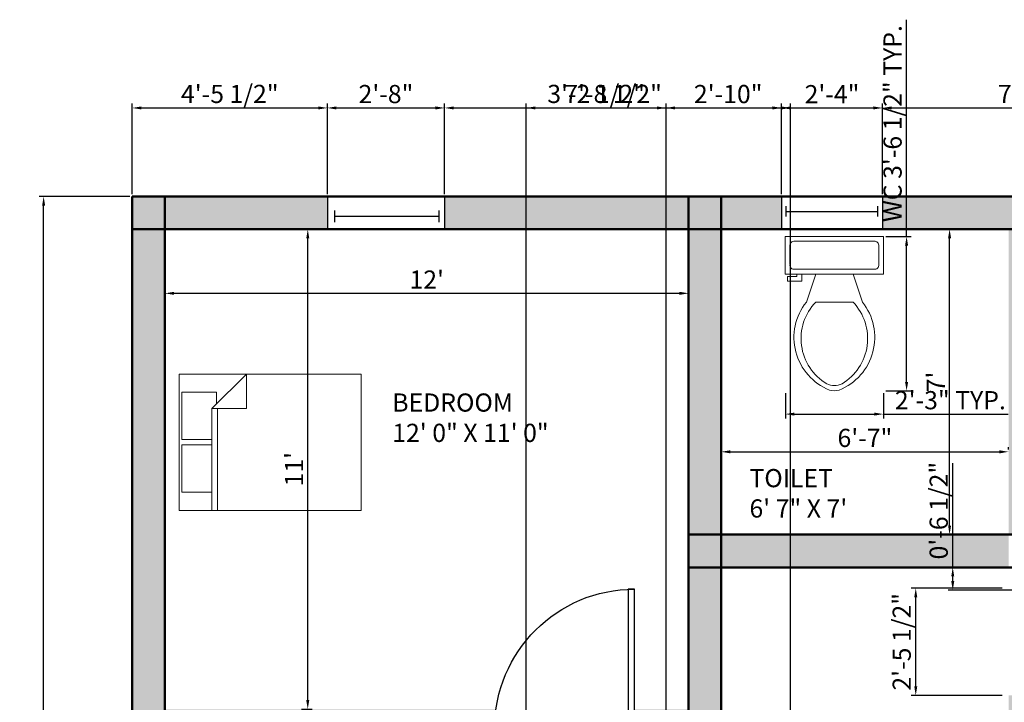
# Model space of a CAD drawing. Units: millimetres. Extents: x 3012 to 3478, y 929 to 1463.
# Tile 3 of 4: x 3012 to 3283, y 1275 to 1463. Entities that reach past the tile are written whole.
import ezdxf

# ---------------------------------------------------------------- set-up
doc = ezdxf.new("R2010")
doc.units = ezdxf.units.MM
for name, color, linetype, lineweight in [('A-ANNO-DIMS', 50, 'Continuous', 18), ('A-AREA-IDEN', 170, 'Continuous', 25), ('A-FLOR-FIXT', 9, 'Continuous', 18), ('A-WALL-PATT', 252, 'Continuous', 13), ('doors', 130, 'Continuous', 25), ('furniture', 80, 'Continuous', 18), ('walls', 10, 'Continuous', 50), ('windows', 40, 'Continuous', 25)]:
    doc.layers.add(name, color=color, linetype=linetype, lineweight=lineweight)
doc.styles.get("Standard").update_dxf_attribs({"font": 'arial.ttf'})
doc.dimstyles.new('ISO-25', dxfattribs={"dimtxt": 5, "dimasz": 2.5, "dimexe": 1.25, "dimexo": 0.625, "dimtad": 1, "dimdec": 0, "dimlunit": 3, "dimtxsty": 'Standard', "dimcen": 2.5, "dimadec": 0, "dimazin": 0, "dimtfac": 1, "dimtdec": 0, "dimtmove": 0, "dimatfit": 3, "dimfxl": 1, "dimarcsym": 0})

# ---------------------------------------------------------------- blocks, each defined once
blk = doc.blocks.new('*U2')
for p, q in [((0, 0), (0, -6)), ((40, 0), (40, -6))]:
    blk.add_line(p, q)
blk.add_lwpolyline([(0, 0), (0, 40), (1.75, 40), (1.75, 0)], close=True)
blk.add_arc((0, 0), 40, 0, 90)
blk = doc.blocks.new('*U4')
for p, q in [((0, 4), (0, 0)), ((36, 4), (36, 0)), ((0, 2), (36, 2))]:
    blk.add_line(p, q)
blk = doc.blocks.new('*U5')
for p, q in [((0, 4), (0, 0)), ((36, 4), (36, 0)), ((0, 2), (36, 2))]:
    blk.add_line(p, q)
blk = doc.blocks.new('Bed - Queen')
for p, q in [((0, -80.00003), (0, 0)), ((0, 0), (59.99999, 0)), ((59.99999, 0), (59.99999, -80.00003)), ((7.99999, -1.2), (28.79998, -1.2)), ((7.99999, -14.4), (7.99999, -1.2)), ((28.79998, -1.2), (28.79998, -14.4)), ((31.19999, -1.2), (51.99999, -1.2)), ((31.19999, -14.4), (31.19999, -1.2)), ((51.99999, -1.2), (51.99999, -16.4)), ((0, -14.4), (44.8, -14.4)), ((44.8, -16.8), (0, -16.8)), ((59.99999, -29.6), (44.8, -14.4)), ((44.8, -14.4), (44.8, -29.6)), ((51.99999, -16.4), (46.79936, -16.4)), ((44.8, -29.6), (59.99999, -29.6)), ((59.99999, -80.00003), (0, -80.00003))]:
    blk.add_line(p, q)
blk = doc.blocks.new('Toilet - top')
for p, q in [((9.5, -6), (9.5, -2)), ((-8, -8.5), (-8, -8)), ((-7, -8), (-7, -9.5)), ((-4, -8), (-6, -14)), ((4, -8), (6, -14)), ((-10, -8.5), (-8, -8.5)), ((-10, -9.5), (-10, -8.5)), ((-7, -9.5), (-10, -9.5)), ((4, -14), (-4, -14))]:
    blk.add_line(p, q)
blk.add_lwpolyline([(10.5, -8), (10.5, 0), (-10.5, 0), (-10.5, -8)], close=True)
for points in [[(-9.5, -2), (-9.5, -6)], [(8.5, -1), (-8.5, -1)], [(-8.5, -7), (8.5, -7)]]:
    blk.add_lwpolyline(points)
for centre, radius, start, end in [((-8.62, -1.88), 0.884, 81.8699, 188.1301), ((8.62, -1.88), 0.884, 351.8699, 98.1301), ((-8.62, -6.12), 0.884, 171.8699, 278.1301), ((8.62, -6.12), 0.884, 261.8699, 8.1301), ((3.52, -21.58), 12.17, 141.4691, 247.9714), ((4.2, -21.82), 11.33, 136.3677, 238.9468), ((-3.52, -21.58), 12.17, 292.0284, 38.5307), ((-4.2, -21.82), 11.33, 301.053, 43.6321), ((0, -27.88), 4, 245.7318, 294.2682), ((0, -29), 4, 254.8605, 285.1395)]:
    blk.add_arc(centre, radius, start, end)
blk = doc.blocks.new('*D12')
at = {"layer": 'A-ANNO-DIMS', "color": 0, "lineweight": -2, "transparency": 16777216}
for p, q in [((3052.21, 1392.44), (3052.21, 1386.56)), ((3196.21, 1392.44), (3196.21, 1386.56)), ((3054.71, 1387.81), (3193.71, 1387.81))]:
    blk.add_line(p, q, dxfattribs=at)
at = {"layer": 'A-ANNO-DIMS', "color": 0, "transparency": 16777216}
for points in [[(3054.71, 1388.22), (3054.71, 1387.39), (3052.21, 1387.81)], [(3193.71, 1388.22), (3193.71, 1387.39), (3196.21, 1387.81)]]:
    blk.add_solid(points, dxfattribs=at)
at = {"layer": 'Defpoints', "color": 0, "transparency": 16777216}
for p in [(3052.21, 1393.06), (3196.21, 1393.06), (3196.21, 1387.81)]:
    blk.add_point(p, dxfattribs=at)
at = {"layer": 'A-ANNO-DIMS', "color": 0, "transparency": 16777216, "insert": (3124.21, 1390.94), "char_height": 5, "attachment_point": 5}
blk.add_mtext("12'", dxfattribs=at)
blk = doc.blocks.new('*D13')
at = {"layer": 'A-ANNO-DIMS', "color": 0, "lineweight": -2, "transparency": 16777216}
for p, q in [((3089.79, 1405.44), (3092.75, 1405.44)), ((3091.5, 1275.94), (3091.5, 1402.94)), ((3089.79, 1273.44), (3092.75, 1273.44))]:
    blk.add_line(p, q, dxfattribs=at)
at = {"layer": 'A-ANNO-DIMS', "color": 0, "transparency": 16777216}
for points in [[(3091.08, 1402.94), (3091.91, 1402.94), (3091.5, 1405.44)], [(3091.08, 1275.94), (3091.91, 1275.94), (3091.5, 1273.44)]]:
    blk.add_solid(points, dxfattribs=at)
at = {"layer": 'Defpoints', "color": 0, "transparency": 16777216}
for p in [(3089.17, 1405.44), (3091.5, 1405.44), (3089.17, 1273.44)]:
    blk.add_point(p, dxfattribs=at)
at = {"layer": 'A-ANNO-DIMS', "color": 0, "transparency": 16777216, "insert": (3088.36, 1339.44), "char_height": 5, "attachment_point": 5, "rotation": 90}
blk.add_mtext("11'", dxfattribs=at)
blk = doc.blocks.new('*D14')
at = {"layer": 'A-ANNO-DIMS', "color": 0, "lineweight": -2, "transparency": 16777216}
for p, q in [((3205.21, 1344.85), (3205.21, 1345.47)), ((3207.71, 1344.22), (3281.71, 1344.22)), ((3284.21, 1344.85), (3284.21, 1345.47))]:
    blk.add_line(p, q, dxfattribs=at)
at = {"layer": 'A-ANNO-DIMS', "color": 0, "transparency": 16777216}
for points in [[(3207.71, 1344.64), (3207.71, 1343.8), (3205.21, 1344.22)], [(3281.71, 1344.64), (3281.71, 1343.8), (3284.21, 1344.22)]]:
    blk.add_solid(points, dxfattribs=at)
at = {"layer": 'Defpoints', "color": 0, "transparency": 16777216}
for p in [(3205.21, 1344.22), (3284.21, 1344.22), (3284.21, 1344.22)]:
    blk.add_point(p, dxfattribs=at)
at = {"layer": 'A-ANNO-DIMS', "color": 0, "transparency": 16777216, "insert": (3244.71, 1347.4), "char_height": 5, "attachment_point": 5}
blk.add_mtext('6\'-7"', dxfattribs=at)
blk = doc.blocks.new('*D15')
at = {"layer": 'A-ANNO-DIMS', "color": 0, "lineweight": -2, "transparency": 16777216}
for p, q in [((3268.62, 1405.44), (3269.24, 1405.44)), ((3267.99, 1323.94), (3267.99, 1402.94)), ((3268.62, 1321.44), (3269.24, 1321.44))]:
    blk.add_line(p, q, dxfattribs=at)
at = {"layer": 'A-ANNO-DIMS', "color": 0, "transparency": 16777216}
for points in [[(3267.58, 1402.94), (3268.41, 1402.94), (3267.99, 1405.44)], [(3267.58, 1323.94), (3268.41, 1323.94), (3267.99, 1321.44)]]:
    blk.add_solid(points, dxfattribs=at)
at = {"layer": 'Defpoints', "color": 0, "transparency": 16777216}
for p in [(3267.99, 1405.44), (3267.99, 1405.44), (3267.99, 1321.44)]:
    blk.add_point(p, dxfattribs=at)
at = {"layer": 'A-ANNO-DIMS', "color": 0, "transparency": 16777216, "insert": (3264.87, 1363.44), "char_height": 5, "attachment_point": 5, "rotation": 90}
blk.add_mtext("7'", dxfattribs=at)
blk = doc.blocks.new('*D32')
at = {"layer": 'A-ANNO-DIMS', "color": 0, "lineweight": -2, "transparency": 16777216}
for p, q in [((3256.17, 1403.4), (3256.17, 1463.07)), ((3250.43, 1403.4), (3257.42, 1403.4)), ((3256.17, 1363.46), (3256.17, 1400.9)), ((3250.43, 1360.96), (3257.42, 1360.96))]:
    blk.add_line(p, q, dxfattribs=at)
at = {"layer": 'A-ANNO-DIMS', "color": 0, "transparency": 16777216}
for points in [[(3255.75, 1400.9), (3256.59, 1400.9), (3256.17, 1403.4)], [(3255.75, 1363.46), (3256.59, 1363.46), (3256.17, 1360.96)]]:
    blk.add_solid(points, dxfattribs=at)
at = {"layer": 'Defpoints', "color": 0, "transparency": 16777216}
for p in [(3249.8, 1403.4), (3256.17, 1403.4), (3249.8, 1360.96)]:
    blk.add_point(p, dxfattribs=at)
at = {"layer": 'A-ANNO-DIMS', "color": 0, "transparency": 16777216, "insert": (3252.96, 1434.49), "char_height": 5, "attachment_point": 5, "rotation": 90}
blk.add_mtext('WC 3\'-6 1/2" TYP.', dxfattribs=at)
blk = doc.blocks.new('*D33')
at = {"layer": 'A-ANNO-DIMS', "color": 0, "lineweight": -2, "transparency": 16777216}
for p, q in [((3222.83, 1360.33), (3222.83, 1353.34)), ((3249.8, 1360.33), (3249.8, 1353.34)), ((3225.33, 1354.59), (3247.3, 1354.59)), ((3249.8, 1354.59), (3284.11, 1354.59))]:
    blk.add_line(p, q, dxfattribs=at)
at = {"layer": 'A-ANNO-DIMS', "color": 0, "transparency": 16777216}
for points in [[(3225.33, 1355.01), (3225.33, 1354.17), (3222.83, 1354.59)], [(3247.3, 1355.01), (3247.3, 1354.17), (3249.8, 1354.59)]]:
    blk.add_solid(points, dxfattribs=at)
at = {"layer": 'Defpoints', "color": 0, "transparency": 16777216}
for p in [(3222.83, 1360.96), (3249.8, 1360.96), (3249.8, 1354.59)]:
    blk.add_point(p, dxfattribs=at)
at = {"layer": 'A-ANNO-DIMS', "color": 0, "transparency": 16777216, "insert": (3268.21, 1357.77), "char_height": 5, "attachment_point": 5}
blk.add_mtext('2\'-3" TYP.', dxfattribs=at)
blk = doc.blocks.new('*D42')
at = {"layer": 'A-ANNO-DIMS', "color": 0, "lineweight": -2, "transparency": 16777216}
for p, q in [((3042.59, 1414.44), (3017.61, 1414.44)), ((3018.86, 959.94), (3018.86, 1411.94)), ((3042.59, 957.44), (3017.61, 957.44))]:
    blk.add_line(p, q, dxfattribs=at)
at = {"layer": 'A-ANNO-DIMS', "color": 0, "transparency": 16777216}
for points in [[(3018.45, 1411.94), (3019.28, 1411.94), (3018.86, 1414.44)], [(3018.45, 959.94), (3019.28, 959.94), (3018.86, 957.44)]]:
    blk.add_solid(points, dxfattribs=at)
at = {"layer": 'Defpoints', "color": 0, "transparency": 16777216}
for p in [(3018.86, 1414.44), (3043.21, 1414.44), (3043.21, 957.44)]:
    blk.add_point(p, dxfattribs=at)
at = {"layer": 'A-ANNO-DIMS', "color": 0, "transparency": 16777216, "insert": (3015.68, 1185.94), "char_height": 5, "attachment_point": 5, "rotation": 90}
blk.add_mtext('38\'-1"', dxfattribs=at)
blk = doc.blocks.new('*D43')
at = {"layer": 'A-ANNO-DIMS', "color": 0, "lineweight": -2, "transparency": 16777216}
for p, q in [((3043.21, 1415.07), (3043.21, 1440.04)), ((3045.71, 1438.79), (3094.39, 1438.79)), ((3096.89, 1415.07), (3096.89, 1440.04))]:
    blk.add_line(p, q, dxfattribs=at)
at = {"layer": 'A-ANNO-DIMS', "color": 0, "transparency": 16777216}
for points in [[(3045.71, 1439.21), (3045.71, 1438.38), (3043.21, 1438.79)], [(3094.39, 1439.21), (3094.39, 1438.38), (3096.89, 1438.79)]]:
    blk.add_solid(points, dxfattribs=at)
at = {"layer": 'Defpoints', "color": 0, "transparency": 16777216}
for p in [(3096.89, 1438.79), (3043.21, 1414.44), (3096.89, 1414.44)]:
    blk.add_point(p, dxfattribs=at)
at = {"layer": 'A-ANNO-DIMS', "color": 0, "transparency": 16777216, "insert": (3070.05, 1442), "char_height": 5, "attachment_point": 5}
blk.add_mtext('4\'-5 1/2"', dxfattribs=at)
blk = doc.blocks.new('*D44')
at = {"layer": 'A-ANNO-DIMS', "color": 0, "lineweight": -2, "transparency": 16777216}
for p, q in [((3096.89, 1415.07), (3096.89, 1440.04)), ((3099.39, 1438.79), (3126.62, 1438.79)), ((3129.12, 1415.07), (3129.12, 1440.04))]:
    blk.add_line(p, q, dxfattribs=at)
at = {"layer": 'A-ANNO-DIMS', "color": 0, "transparency": 16777216}
for points in [[(3099.39, 1439.21), (3099.39, 1438.38), (3096.89, 1438.79)], [(3126.62, 1439.21), (3126.62, 1438.38), (3129.12, 1438.79)]]:
    blk.add_solid(points, dxfattribs=at)
at = {"layer": 'Defpoints', "color": 0, "transparency": 16777216}
for p in [(3129.12, 1438.79), (3096.89, 1414.44), (3129.12, 1414.44)]:
    blk.add_point(p, dxfattribs=at)
at = {"layer": 'A-ANNO-DIMS', "color": 0, "transparency": 16777216, "insert": (3113, 1441.97), "char_height": 5, "attachment_point": 5}
blk.add_mtext('2\'-8"', dxfattribs=at)
blk = doc.blocks.new('*D45')
at = {"layer": 'A-ANNO-DIMS', "color": 0, "lineweight": -2, "transparency": 16777216}
for p, q in [((3129.12, 1415.07), (3129.12, 1440.04)), ((3131.62, 1438.79), (3219.29, 1438.79)), ((3221.79, 1415.07), (3221.79, 1440.04))]:
    blk.add_line(p, q, dxfattribs=at)
at = {"layer": 'A-ANNO-DIMS', "color": 0, "transparency": 16777216}
for points in [[(3131.62, 1439.21), (3131.62, 1438.38), (3129.12, 1438.79)], [(3219.29, 1439.21), (3219.29, 1438.38), (3221.79, 1438.79)]]:
    blk.add_solid(points, dxfattribs=at)
at = {"layer": 'Defpoints', "color": 0, "transparency": 16777216}
for p in [(3221.79, 1438.79), (3129.12, 1414.44), (3221.79, 1414.44)]:
    blk.add_point(p, dxfattribs=at)
at = {"layer": 'A-ANNO-DIMS', "color": 0, "transparency": 16777216, "insert": (3175.46, 1442), "char_height": 5, "attachment_point": 5}
blk.add_mtext('7\'-8 1/2"', dxfattribs=at)
blk = doc.blocks.new('*D46')
at = {"layer": 'A-ANNO-DIMS', "color": 0, "lineweight": -2, "transparency": 16777216}
for p, q in [((3221.79, 1415.07), (3221.79, 1440.04)), ((3224.29, 1438.79), (3247.05, 1438.79)), ((3249.55, 1415.07), (3249.55, 1440.04))]:
    blk.add_line(p, q, dxfattribs=at)
at = {"layer": 'A-ANNO-DIMS', "color": 0, "transparency": 16777216}
for points in [[(3224.29, 1439.21), (3224.29, 1438.38), (3221.79, 1438.79)], [(3247.05, 1439.21), (3247.05, 1438.38), (3249.55, 1438.79)]]:
    blk.add_solid(points, dxfattribs=at)
at = {"layer": 'Defpoints', "color": 0, "transparency": 16777216}
for p in [(3249.55, 1438.79), (3221.79, 1414.44), (3249.55, 1414.44)]:
    blk.add_point(p, dxfattribs=at)
at = {"layer": 'A-ANNO-DIMS', "color": 0, "transparency": 16777216, "insert": (3235.67, 1441.93), "char_height": 5, "attachment_point": 5}
blk.add_mtext('2\'-4"', dxfattribs=at)
blk = doc.blocks.new('*D47')
at = {"layer": 'A-ANNO-DIMS', "color": 0, "lineweight": -2, "transparency": 16777216}
for p, q in [((3249.55, 1415.07), (3249.55, 1440.04)), ((3252.05, 1438.79), (3337.37, 1438.79)), ((3339.87, 1415.07), (3339.87, 1440.04))]:
    blk.add_line(p, q, dxfattribs=at)
at = {"layer": 'A-ANNO-DIMS', "color": 0, "transparency": 16777216}
for points in [[(3252.05, 1439.21), (3252.05, 1438.38), (3249.55, 1438.79)], [(3337.37, 1439.21), (3337.37, 1438.38), (3339.87, 1438.79)]]:
    blk.add_solid(points, dxfattribs=at)
at = {"layer": 'Defpoints', "color": 0, "transparency": 16777216}
for p in [(3339.87, 1438.79), (3249.55, 1414.44), (3339.87, 1414.44)]:
    blk.add_point(p, dxfattribs=at)
at = {"layer": 'A-ANNO-DIMS', "color": 0, "transparency": 16777216, "insert": (3294.71, 1442), "char_height": 5, "attachment_point": 5}
blk.add_mtext('7\'-6 1/2"', dxfattribs=at)
blk = doc.blocks.new('*D59')
at = {"layer": 'A-ANNO-DIMS', "color": 0, "lineweight": -2, "transparency": 16777216}
for p, q in [((3282.42, 1306.73), (3257.44, 1306.73)), ((3258.69, 1279.72), (3258.69, 1304.23)), ((3282.42, 1277.22), (3257.44, 1277.22))]:
    blk.add_line(p, q, dxfattribs=at)
at = {"layer": 'A-ANNO-DIMS', "color": 0, "transparency": 16777216}
for points in [[(3258.28, 1304.23), (3259.11, 1304.23), (3258.69, 1306.73)], [(3258.28, 1279.72), (3259.11, 1279.72), (3258.69, 1277.22)]]:
    blk.add_solid(points, dxfattribs=at)
at = {"layer": 'Defpoints', "color": 0, "transparency": 16777216}
for p in [(3258.69, 1306.73), (3283.04, 1306.73), (3283.04, 1277.22)]:
    blk.add_point(p, dxfattribs=at)
at = {"layer": 'A-ANNO-DIMS', "color": 0, "transparency": 16777216, "insert": (3255.48, 1291.97), "char_height": 5, "attachment_point": 5, "rotation": 90}
blk.add_mtext('2\'-5 1/2"', dxfattribs=at)
blk = doc.blocks.new('*D60')
at = {"layer": 'A-ANNO-DIMS', "color": 0, "lineweight": -2, "transparency": 16777216}
for p, q in [((3268.86, 1312.44), (3268.86, 1341.13)), ((3292.59, 1312.44), (3267.61, 1312.44)), ((3268.86, 1308.66), (3268.86, 1309.94)), ((3292.59, 1306.16), (3267.61, 1306.16))]:
    blk.add_line(p, q, dxfattribs=at)
at = {"layer": 'A-ANNO-DIMS', "color": 0, "transparency": 16777216}
for points in [[(3268.45, 1309.94), (3269.28, 1309.94), (3268.86, 1312.44)], [(3268.45, 1308.66), (3269.28, 1308.66), (3268.86, 1306.16)]]:
    blk.add_solid(points, dxfattribs=at)
at = {"layer": 'Defpoints', "color": 0, "transparency": 16777216}
for p in [(3268.86, 1312.44), (3293.21, 1312.44), (3293.21, 1306.16)]:
    blk.add_point(p, dxfattribs=at)
at = {"layer": 'A-ANNO-DIMS', "color": 0, "transparency": 16777216, "insert": (3265.65, 1328.04), "char_height": 5, "attachment_point": 5, "rotation": 90}
blk.add_mtext('0\'-6 1/2"', dxfattribs=at)
blk = doc.blocks.new('*D61')
at = {"layer": 'A-ANNO-DIMS', "color": 0, "lineweight": -2, "transparency": 16777216}
for p, q in [((3151.56, 1133.07), (3151.56, 1440.04)), ((3154.06, 1438.79), (3187.51, 1438.79)), ((3190.01, 1133.07), (3190.01, 1440.04))]:
    blk.add_line(p, q, dxfattribs=at)
at = {"layer": 'A-ANNO-DIMS', "color": 0, "transparency": 16777216}
for points in [[(3154.06, 1439.21), (3154.06, 1438.38), (3151.56, 1438.79)], [(3187.51, 1439.21), (3187.51, 1438.38), (3190.01, 1438.79)]]:
    blk.add_solid(points, dxfattribs=at)
at = {"layer": 'Defpoints', "color": 0, "transparency": 16777216}
for p in [(3190.01, 1438.79), (3151.56, 1132.44), (3190.01, 1132.44)]:
    blk.add_point(p, dxfattribs=at)
at = {"layer": 'A-ANNO-DIMS', "color": 0, "transparency": 16777216, "insert": (3170.79, 1442), "char_height": 5, "attachment_point": 5}
blk.add_mtext('3\'-2 1/2"', dxfattribs=at)
blk = doc.blocks.new('*D62')
at = {"layer": 'A-ANNO-DIMS', "color": 0, "lineweight": -2, "transparency": 16777216}
for p, q in [((3190.01, 1133.07), (3190.01, 1440.04)), ((3192.51, 1438.79), (3221.71, 1438.79)), ((3224.21, 1133.07), (3224.21, 1440.04))]:
    blk.add_line(p, q, dxfattribs=at)
at = {"layer": 'A-ANNO-DIMS', "color": 0, "transparency": 16777216}
for points in [[(3192.51, 1439.21), (3192.51, 1438.38), (3190.01, 1438.79)], [(3221.71, 1439.21), (3221.71, 1438.38), (3224.21, 1438.79)]]:
    blk.add_solid(points, dxfattribs=at)
at = {"layer": 'Defpoints', "color": 0, "transparency": 16777216}
for p in [(3224.21, 1438.79), (3190.01, 1132.44), (3224.21, 1132.44)]:
    blk.add_point(p, dxfattribs=at)
at = {"layer": 'A-ANNO-DIMS', "color": 0, "transparency": 16777216, "insert": (3207.11, 1441.97), "char_height": 5, "attachment_point": 5}
blk.add_mtext('2\'-10"', dxfattribs=at)

msp = doc.modelspace()

# ---------------------------------------------------------------- hatches: boundary and pattern name
at = {"layer": 'A-WALL-PATT'}
h = msp.add_hatch(color=256, dxfattribs=at)
h.dxf.hatch_style = 1
h.paths.add_polyline_path([(3052.21, 1405.44), (3043.21, 1405.44), (3043.21, 1273.44), (3052.21, 1273.44)])
h.paths.add_polyline_path([(3052.21, 1273.44), (3043.21, 1273.44), (3043.21, 1264.44), (3052.21, 1264.44)])
h.paths.add_polyline_path([(3052.21, 1264.44), (3043.21, 1264.44), (3043.21, 1132.44), (3052.21, 1132.44)])
h.paths.add_polyline_path([(3116.21, 1273.44), (3052.21, 1273.44), (3052.21, 1264.44), (3116.21, 1264.44)])
h.paths.add_polyline_path([(3125.21, 1273.44), (3116.21, 1273.44), (3116.21, 1264.44), (3125.21, 1264.44)])
h.paths.add_polyline_path([(3143.26, 1273.44), (3125.21, 1273.44), (3125.21, 1264.44), (3142.87, 1264.44), (3142.87, 1268, -0.035543)])
h.paths.add_polyline_path([(3052.21, 1414.44), (3043.21, 1414.44), (3043.21, 1405.44), (3052.21, 1405.44)])
h.paths.add_polyline_path([(3096.89, 1414.44), (3052.21, 1414.44), (3052.21, 1405.44), (3096.89, 1405.44)])
h.paths.add_polyline_path([(3196.21, 1414.44), (3129.12, 1414.44), (3129.12, 1405.44), (3196.21, 1405.44)])
h.paths.add_polyline_path([(3205.21, 1414.44), (3196.21, 1414.44), (3196.21, 1405.44), (3205.21, 1405.44)])
h.paths.add_polyline_path([(3205.21, 1405.44), (3196.21, 1405.44), (3196.21, 1321.44), (3205.21, 1321.44)])
h.paths.add_polyline_path([(3205.21, 1321.44), (3196.21, 1321.44), (3196.21, 1312.44), (3205.21, 1312.44)])
h.paths.add_polyline_path([(3205.21, 1312.44), (3196.21, 1312.44), (3196.21, 1273.44), (3205.21, 1273.44)])
h.paths.add_polyline_path([(3284.21, 1321.44), (3205.21, 1321.44), (3205.21, 1312.44), (3284.21, 1312.44)])
h.paths.add_polyline_path([(3205.21, 1273.44), (3196.21, 1273.44), (3196.21, 1264.44), (3205.21, 1264.44)])
h.paths.add_polyline_path([(3196.21, 1273.44), (3181.32, 1273.44), (3181.32, 1268), (3181.32, 1264.44), (3196.21, 1264.44)])
h.paths.add_polyline_path([(3293.21, 1405.44), (3284.21, 1405.44), (3284.21, 1321.44), (3293.21, 1321.44)])
h.paths.add_polyline_path([(3293.21, 1414.44), (3284.21, 1414.44), (3284.21, 1405.44), (3293.21, 1405.44)])
h.paths.add_polyline_path([(3284.21, 1414.44), (3249.55, 1414.44), (3249.55, 1405.44), (3284.21, 1405.44)])
h.paths.add_polyline_path([(3221.79, 1414.44), (3205.21, 1414.44), (3205.21, 1405.44), (3221.79, 1405.44)])
h.paths.add_polyline_path([(3339.87, 1414.44), (3293.21, 1414.44), (3293.21, 1405.44), (3339.87, 1405.44)])
h.paths.add_polyline_path([(3437.21, 1414.44), (3373.17, 1414.44), (3373.17, 1405.44), (3437.21, 1405.44)])
h.paths.add_polyline_path([(3446.21, 1414.44), (3437.21, 1414.44), (3437.21, 1405.44), (3446.21, 1405.44)])
h.paths.add_polyline_path([(3446.21, 1405.44), (3437.21, 1405.44), (3437.21, 1273.44), (3446.21, 1273.44)])
h.paths.add_polyline_path([(3437.21, 1273.44), (3293.21, 1273.44), (3293.21, 1264.44), (3437.21, 1264.44)])
h.paths.add_polyline_path([(3446.21, 1273.44), (3437.21, 1273.44), (3437.21, 1264.44), (3446.21, 1264.44)])
h.paths.add_polyline_path([(3446.21, 1264.44), (3437.21, 1264.44), (3437.21, 1249.83), (3445.52, 1249.83), (3446.21, 1249.83)])
h.paths.add_polyline_path([(3293.21, 1264.44), (3284.21, 1264.44), (3284.21, 1132.44), (3293.21, 1132.44)])
h.paths.add_polyline_path([(3293.21, 1273.44), (3284.21, 1273.44), (3284.21, 1264.44), (3293.21, 1264.44)])
h.paths.add_polyline_path([(3293.21, 1277.22), (3287.47, 1277.22), (3284.21, 1277.22), (3284.21, 1273.44), (3293.21, 1273.44)])
h.paths.add_polyline_path([(3125.21, 1213.86), (3116.21, 1213.86), (3116.21, 1184.42), (3125.21, 1184.42)])
h.paths.add_polyline_path([(3125.21, 1264.44), (3116.21, 1264.44), (3116.21, 1245.36), (3125.21, 1245.36)])
h.paths.add_polyline_path([(3125.21, 1151.51), (3116.21, 1151.51), (3116.21, 1132.44), (3125.21, 1132.44)])
h.paths.add_polyline_path([(3125.21, 1132.44), (3116.21, 1132.44), (3116.21, 1123.44), (3125.21, 1123.44)])
h.paths.add_polyline_path([(3151.56, 1127.56), (3151.56, 1132.44), (3125.21, 1132.44), (3125.21, 1123.44), (3151.56, 1123.44)])
h.paths.add_polyline_path([(3116.21, 1132.44), (3052.21, 1132.44), (3052.21, 1123.44), (3116.21, 1123.44)])
h.paths.add_polyline_path([(3052.21, 1132.44), (3043.21, 1132.44), (3043.21, 1123.44), (3052.21, 1123.44)])
h.paths.add_polyline_path([(3052.21, 1123.44), (3043.21, 1123.44), (3043.21, 966.44), (3052.21, 966.44)])
h.paths.add_polyline_path([(3097.57, 966.44), (3052.21, 966.44), (3052.21, 957.44), (3097.57, 957.44)])
h.paths.add_polyline_path([(3052.21, 966.44), (3043.21, 966.44), (3043.21, 957.44), (3052.21, 957.44)])
h.paths.add_polyline_path([(3215.21, 966.44), (3131.05, 966.44), (3131.05, 957.44), (3215.21, 957.44)])
h.paths.add_polyline_path([(3224.21, 966.44), (3215.21, 966.44), (3215.21, 957.44), (3224.21, 957.44)])
h.paths.add_polyline_path([(3224.21, 1004.97, -0.051409), (3218.39, 1004.37), (3215.21, 1004.37), (3215.21, 966.44), (3224.21, 966.44)])
h.paths.add_polyline_path([(3239.46, 966.44), (3224.21, 966.44), (3224.21, 957.44), (3239.46, 957.44)])
h.paths.add_polyline_path([(3344.91, 966.44), (3266.71, 966.44), (3266.71, 957.44), (3344.91, 957.44)])
h.paths.add_polyline_path([(3293.21, 1018.44), (3284.21, 1018.44), (3284.21, 966.44), (3293.21, 966.44)])
h.paths.add_polyline_path([(3293.21, 1027.44), (3284.21, 1027.44), (3284.21, 1018.44), (3293.21, 1018.44)])
h.paths.add_polyline_path([(3293.21, 1074.44), (3284.21, 1074.44), (3284.21, 1027.44), (3293.21, 1027.44)])
h.paths.add_polyline_path([(3224.21, 1074.44), (3215.21, 1074.44), (3215.21, 1032.91), (3218.39, 1032.91), (3224.21, 1032.91)])
h.paths.add_polyline_path([(3224.21, 1123.44), (3215.21, 1123.44), (3215.21, 1083.44), (3224.21, 1083.44)])
h.paths.add_polyline_path([(3224.21, 1083.44), (3215.21, 1083.44), (3215.21, 1074.44), (3224.21, 1074.44)])
h.paths.add_polyline_path([(3284.21, 1083.44), (3224.21, 1083.44), (3224.21, 1074.44), (3284.21, 1074.44)])
h.paths.add_polyline_path([(3293.21, 1083.44), (3284.21, 1083.44), (3284.21, 1074.44), (3293.21, 1074.44)])
h.paths.add_polyline_path([(3215.21, 1132.44), (3190.01, 1132.44), (3190.01, 1127.56, -0.026825), (3189.79, 1123.44), (3215.21, 1123.44)])
h.paths.add_polyline_path([(3224.21, 1132.44), (3215.21, 1132.44), (3215.21, 1123.44), (3224.21, 1123.44)])
h.paths.add_polyline_path([(3437.21, 1132.44), (3293.21, 1132.44), (3293.21, 1123.44), (3437.21, 1123.44)])
h.paths.add_polyline_path([(3293.21, 1132.44), (3284.21, 1132.44), (3284.21, 1123.44), (3293.21, 1123.44)])
h.paths.add_polyline_path([(3446.21, 1132.44), (3437.21, 1132.44), (3437.21, 1123.44), (3446.21, 1123.44)])
h.paths.add_polyline_path([(3446.21, 1123.44), (3437.21, 1123.44), (3437.21, 1027.44), (3446.21, 1027.44)])
h.paths.add_polyline_path([(3446.21, 1221.29), (3445.52, 1221.29, -0.074007), (3437.21, 1222.53), (3437.21, 1132.44), (3446.21, 1132.44)])
h.paths.add_polyline_path([(3446.21, 1018.44), (3437.21, 1018.44), (3437.21, 966.44), (3446.21, 966.44)])
h.paths.add_polyline_path([(3446.21, 1027.44), (3437.21, 1027.44), (3437.21, 1018.44), (3446.21, 1018.44)])
h.paths.add_polyline_path([(3437.21, 1027.44), (3389.3, 1027.44), (3389.3, 1025.95), (3389.3, 1018.44), (3437.21, 1018.44)])
h.paths.add_polyline_path([(3360.77, 1025.95), (3360.77, 1027.44), (3293.21, 1027.44), (3293.21, 1018.44), (3361.77, 1018.44, -0.066618)])
h.paths.add_polyline_path([(3437.21, 966.44), (3375.49, 966.44), (3375.49, 957.44), (3437.21, 957.44)])
h.paths.add_polyline_path([(3446.21, 966.44), (3437.21, 966.44), (3437.21, 957.44), (3446.21, 957.44)])

# ---------------------------------------------------------------- linework, layer by layer
at = {"layer": 'walls'}
for p, q in [((3043.21, 1414.44), (3043.21, 957.44)), ((3043.21, 1414.44), (3446.21, 1414.44)), ((3052.21, 1414.44), (3052.21, 957.44)), ((3196.21, 1414.44), (3196.21, 1264.44)), ((3205.21, 1414.44), (3205.21, 1264.44)), ((3043.21, 1405.44), (3446.21, 1405.44)), ((3196.21, 1321.44), (3293.21, 1321.44)), ((3196.21, 1312.44), (3293.21, 1312.44))]:
    msp.add_line(p, q, dxfattribs=at)
at = {"layer": 'windows'}
for p, q in [((3096.89, 1414.44), (3096.89, 1405.44)), ((3129.12, 1414.44), (3129.12, 1405.44)), ((3221.79, 1414.44), (3221.79, 1405.44)), ((3249.55, 1414.44), (3249.55, 1405.44))]:
    msp.add_line(p, q, dxfattribs=at)

# ---------------------------------------------------------------- block references
at = {"layer": 'A-FLOR-FIXT', "xscale": 1.284488889705511, "yscale": 1.284488889705511, "zscale": 1.284488889705511}
msp.add_blockref('Toilet - top', (3236.31, 1403.4), dxfattribs=at)
at = {"layer": 'doors', "xscale": -0.9611587719732299, "yscale": 0.9611587719732299, "zscale": 0.9611587719732299}
msp.add_blockref('*U2', (3181.32, 1268), dxfattribs=at)
at = {"layer": 'furniture', "xscale": 0.625172702944318, "yscale": 0.625172702944318, "zscale": 0.625172702944318, "rotation": 89.99999999999999}
msp.add_blockref('Bed - Queen', (3056.13, 1328.09), dxfattribs=at)
at = {"layer": 'windows'}
for name, p, xscale, yscale, zscale in [('*U5', (3223, 1408.95), 0.6985876539182364, 0.6985876539182364, 0.6985876539182364), ('*U4', (3098.83, 1407.41), 0.7972415233030418, 0.7972415233030418, 0.7972415233030418)]:
    msp.add_blockref(name, p, dxfattribs=dict(at, xscale=xscale, yscale=yscale, zscale=zscale))

# ---------------------------------------------------------------- texts
at = {"layer": 'A-AREA-IDEN', "char_height": 5, "attachment_point": 1}
for s, width, insert in [('BEDROOM \\P12\' 0" X 11\' 0"', 81.4708, (3114.74, 1360.27)), ('TOILET \\P6\' 7" X 7\'', 50.805, (3212.96, 1339.48))]:
    msp.add_mtext_dynamic_manual_height_columns(s, width=width, gutter_width=12.5, heights=[0], dxfattribs=dict(at, insert=insert))

# ---------------------------------------------------------------- dimensions: what is measured, and where the dimension line sits
at = {"layer": 'A-ANNO-DIMS'}
dim = msp.add_linear_dim(base=(3256.17, 1403.4), p1=(3249.8, 1360.96), p2=(3249.8, 1403.4), angle=90, text='WC <> TYP.', dimstyle='ISO-25', override={"dimdec": 1, "dimlfac": 1, "dimrnd": 0, "dimzin": 1, "dimdsep": 46, "dimlunit": 4, "dimfrac": 2}, dxfattribs=at)
dim.commit()
dim.dimension.update_dxf_attribs({"geometry": '*D32', "text_midpoint": (3252.96, 1434.49)})
for base, p1, p2, override, picture, middle in [((3096.89, 1438.79), (3043.21, 1414.44), (3096.89, 1414.44), {"dimdec": 1, "dimlfac": 1, "dimrnd": 0, "dimzin": 1, "dimdsep": 46, "dimlunit": 4, "dimfrac": 2}, '*D43', (3070.05, 1442)), ((3221.79, 1438.79), (3129.12, 1414.44), (3221.79, 1414.44), {"dimdec": 1, "dimlfac": 1, "dimrnd": 0, "dimzin": 1, "dimdsep": 46, "dimlunit": 4, "dimfrac": 2}, '*D45', (3175.46, 1442)), ((3190.0089, 1438.7917), (3151.5625, 1132.4417), (3190.0089, 1132.4417), {"dimdec": 1, "dimlfac": 1, "dimrnd": 0, "dimzin": 1, "dimdsep": 46, "dimlunit": 4, "dimfrac": 2}, '*D61', (3170.7857, 1442.0037)), ((3339.87, 1438.79), (3249.55, 1414.44), (3339.87, 1414.44), {"dimdec": 1, "dimlfac": 1, "dimrnd": 0, "dimzin": 1, "dimdsep": 46, "dimlunit": 4, "dimfrac": 2}, '*D47', (3294.71, 1442)), ((3129.12, 1438.79), (3096.89, 1414.44), (3129.12, 1414.44), {"dimdec": 1, "dimlfac": 1, "dimrnd": 0, "dimzin": 1, "dimdsep": 46, "dimlunit": 4, "dimfrac": 2}, '*D44', (3113, 1441.97)), ((3224.21, 1438.79), (3190.01, 1132.44), (3224.21, 1132.44), {"dimdec": 1, "dimlfac": 1, "dimrnd": 0, "dimzin": 1, "dimdsep": 46, "dimlunit": 4, "dimfrac": 2}, '*D62', (3207.11, 1441.97)), ((3249.55, 1438.79), (3221.79, 1414.44), (3249.55, 1414.44), {"dimdec": 1, "dimlfac": 1, "dimrnd": 0, "dimzin": 1, "dimdsep": 46, "dimlunit": 4, "dimfrac": 2}, '*D46', (3235.67, 1441.93)), ((3196.21, 1387.81), (3052.21, 1393.06), (3196.21, 1393.06), {"dimclrd": 0, "dimclre": 0, "dimclrt": 0}, '*D12', (3124.21, 1390.94)), ((3284.21, 1344.22), (3205.21, 1344.22), (3284.21, 1344.22), {"dimclrd": 0, "dimclre": 0, "dimclrt": 0}, '*D14', (3244.71, 1347.4))]:
    dim = msp.add_linear_dim(base=base, p1=p1, p2=p2, dimstyle='ISO-25', override=override, dxfattribs=at)
    dim.commit()
    dim.dimension.update_dxf_attribs({"geometry": picture, "text_midpoint": middle})
for base, p1, p2, override, picture, middle in [((3018.86, 1414.44), (3043.21, 957.44), (3043.21, 1414.44), {"dimdec": 1, "dimlfac": 1, "dimrnd": 0, "dimzin": 1, "dimdsep": 46, "dimlunit": 4, "dimfrac": 2}, '*D42', (3015.68, 1185.94)), ((3091.5, 1405.44), (3089.17, 1273.44), (3089.17, 1405.44), {"dimclrd": 0, "dimclre": 0, "dimclrt": 0}, '*D13', (3088.36, 1339.44)), ((3267.99, 1405.44), (3267.99, 1321.44), (3267.99, 1405.44), {"dimclrd": 0, "dimclre": 0, "dimclrt": 0}, '*D15', (3264.87, 1363.44)), ((3268.86, 1312.44), (3293.21, 1306.16), (3293.21, 1312.44), {"dimdec": 1, "dimlfac": 1, "dimrnd": 0, "dimzin": 1, "dimdsep": 46, "dimlunit": 4, "dimfrac": 2}, '*D60', (3265.65, 1328.04)), ((3258.69, 1306.73), (3283.04, 1277.22), (3283.04, 1306.73), {"dimdec": 1, "dimlfac": 1, "dimrnd": 0, "dimzin": 1, "dimdsep": 46, "dimlunit": 4, "dimfrac": 2}, '*D59', (3255.48, 1291.97))]:
    dim = msp.add_linear_dim(base=base, p1=p1, p2=p2, angle=90, dimstyle='ISO-25', override=override, dxfattribs=at)
    dim.commit()
    dim.dimension.update_dxf_attribs({"geometry": picture, "text_midpoint": middle})
dim = msp.add_linear_dim(base=(3249.8, 1354.59), p1=(3222.83, 1360.96), p2=(3249.8, 1360.96), text='<> TYP.', dimstyle='ISO-25', override={"dimdec": 1, "dimlfac": 1, "dimrnd": 0, "dimzin": 1, "dimdsep": 46, "dimlunit": 4, "dimfrac": 2}, dxfattribs=at)
dim.commit()
dim.dimension.update_dxf_attribs({"geometry": '*D33', "text_midpoint": (3268.21, 1357.77)})

doc.saveas('drawing.dxf')
